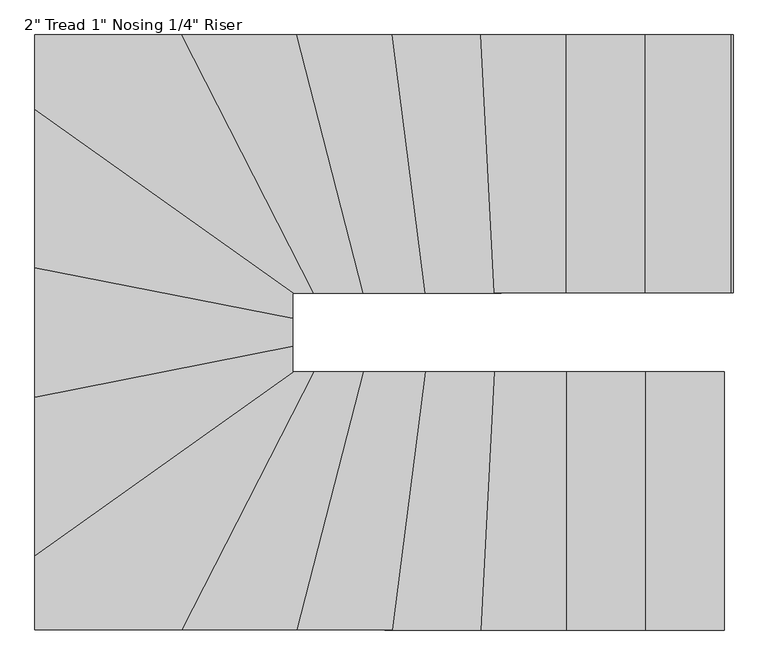
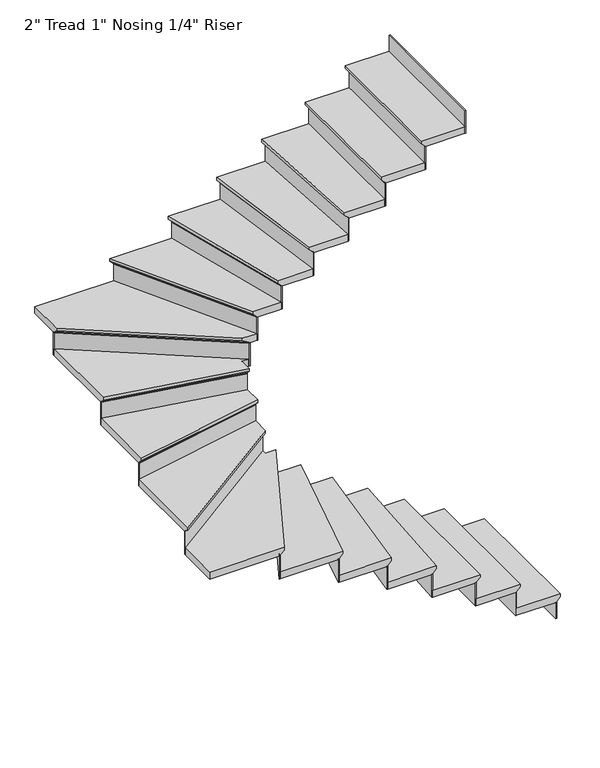
"""IFC4 building model written with IfcOpenShell, lengths in millimetres: stair flight geometry."""

from ifc_helpers import new_model, si_unit, origin, place, context, project, spatial, faceted_brep, source, transform, mapped, element, save


def stair_flight_b82eb699(model_context):
    return source(origin(), model_context, "Body", "Brep", [
        faceted_brep([(-8198.7117747, 8373.1716937, 150.2833333), (-8198.7117747, 8373.1716937, 169.3333333), (-8198.7117747, 7458.7716937, 169.3333333), (-8198.7117747, 7458.7716937, 150.2833333), (-8224.1117747, 8373.1716937, 124.8833333), (-8224.1117747, 7458.7716937, 124.8833333), (-8503.5117747, 8373.1716937, 169.3333333), (-8503.5117747, 7458.7716937, 169.3333333), (-8224.1117747, 7458.7716937, 118.5333333), (-8503.5117747, 7458.7716937, 118.5333333), (-8503.5117747, 8373.1716937, 118.5333333), (-8224.1117747, 8373.1716937, 118.5333333)], [[[0, 1, 2, 3]], [[4, 0, 3, 5]], [[2, 1, 6, 7]], [[8, 9, 10, 11]], [[2, 7, 9, 8, 5, 3]], [[8, 11, 4, 5]], [[6, 1, 0, 4, 11, 10]], [[7, 6, 10, 9]]]),
        faceted_brep([(-8224.1117747, 8373.1716937, 118.5333333), (-8224.1117747, 8373.1716937, 0.0), (-8230.4617747, 8373.1716937, 0.0), (-8230.4617747, 8373.1716937, 118.5333333), (-8224.1117747, 7458.7716937, 118.5333333), (-8230.4617747, 7458.7716937, 118.5333333), (-8230.4617747, 7458.7716937, 0.0), (-8224.1117747, 7458.7716937, 0.0)], [[[0, 1, 2, 3]], [[4, 5, 6, 7]], [[1, 0, 4, 7]], [[2, 1, 7, 6]], [[3, 2, 6, 5]], [[0, 3, 5, 4]]]),
        faceted_brep([(-8503.5117747, 8373.1716937, 287.8666667), (-8503.5117747, 8373.1716937, 118.5333333), (-8509.8617747, 8373.1716937, 118.5333333), (-8509.8617747, 8373.1716937, 287.8666667), (-8503.5117747, 7458.7716937, 287.8666667), (-8509.8617747, 7458.7716937, 287.8666667), (-8509.8617747, 7458.7716937, 118.5333333), (-8503.5117747, 7458.7716937, 118.5333333)], [[[0, 1, 2, 3]], [[4, 5, 6, 7]], [[1, 0, 4, 7]], [[2, 1, 7, 6]], [[3, 2, 6, 5]], [[0, 3, 5, 4]]]),
        faceted_brep([(-8478.1117747, 7458.7716937, 338.6666667), (-8478.1117747, 8373.1716937, 338.6666667), (-8782.9117747, 8373.1716937, 338.6666667), (-8782.9117747, 7458.7716937, 338.6666667), (-8503.5117747, 7458.7716937, 287.8666667), (-8782.9117747, 7458.7716937, 287.8666667), (-8782.9117747, 8373.1716937, 287.8666667), (-8503.5117747, 8373.1716937, 287.8666667), (-8503.5117747, 7458.7716937, 294.2166667), (-8478.1117747, 7458.7716937, 319.6166667), (-8503.5117747, 8373.1716937, 294.2166667), (-8478.1117747, 8373.1716937, 319.6166667)], [[[0, 1, 2, 3]], [[4, 5, 6, 7]], [[0, 3, 5, 4, 8, 9]], [[4, 7, 10, 8]], [[2, 1, 11, 10, 7, 6]], [[3, 2, 6, 5]], [[11, 1, 0, 9]], [[10, 11, 9, 8]]]),
        faceted_brep([(-8782.9117747, 8373.1716937, 457.2), (-8782.9117747, 8373.1716937, 287.8666667), (-8789.2617747, 8373.1716937, 287.8666667), (-8789.2617747, 8373.1716937, 457.2), (-8782.9117747, 7458.7716937, 457.2), (-8789.2617747, 7458.7716937, 457.2), (-8789.2617747, 7458.7716937, 287.8666667), (-8782.9117747, 7458.7716937, 287.8666667)], [[[0, 1, 2, 3]], [[4, 5, 6, 7]], [[1, 0, 4, 7]], [[2, 1, 7, 6]], [[3, 2, 6, 5]], [[0, 3, 5, 4]]]),
        faceted_brep([(-8757.5117747, 7458.7716937, 508.0), (-8757.5117747, 8373.1716937, 508.0), (-9038.5789362, 8373.1716937, 508.0), (-9086.1132066, 7458.7716937, 508.0), (-8782.9117747, 7458.7716937, 457.2), (-9086.1132066, 7458.7716937, 457.2), (-9038.5789362, 8373.1716937, 457.2), (-8782.9117747, 8373.1716937, 457.2), (-8782.9117747, 7458.7716937, 463.55), (-8757.5117747, 7458.7716937, 488.95), (-8782.9117747, 8373.1716937, 463.55), (-8757.5117747, 8373.1716937, 488.95)], [[[0, 1, 2, 3]], [[4, 5, 6, 7]], [[0, 3, 5, 4, 8, 9]], [[4, 7, 10, 8]], [[2, 1, 11, 10, 7, 6]], [[3, 2, 6, 5]], [[11, 1, 0, 9]], [[10, 11, 9, 8]]]),
        faceted_brep([(-9038.5789362, 8373.1716937, 626.5333333), (-9038.5789362, 8373.1716937, 457.2), (-9044.9375104, 8373.1716937, 457.2), (-9044.9375104, 8373.1716937, 626.5333333), (-9086.1132066, 7458.7716937, 626.5333333), (-9092.4717808, 7458.7716937, 626.5333333), (-9092.4717808, 7458.7716937, 457.2), (-9086.1132066, 7458.7716937, 457.2)], [[[0, 1, 2, 3]], [[4, 5, 6, 7]], [[1, 0, 4, 7]], [[2, 1, 7, 6]], [[3, 2, 6, 5]], [[0, 3, 5, 4]]]),
        faceted_brep([(-9060.67891, 7458.7716937, 677.3333333), (-9013.1446395, 8373.1716937, 677.3333333), (-9282.745636, 8373.1716937, 677.3333333), (-9401.1016877, 7458.7716937, 677.3333333), (-9086.1132066, 7458.7716937, 626.5333333), (-9401.1016877, 7458.7716937, 626.5333333), (-9282.745636, 8373.1716937, 626.5333333), (-9038.5789362, 8373.1716937, 626.5333333), (-9086.1132066, 7458.7716937, 632.8833333), (-9060.67891, 7458.7716937, 658.2833333), (-9038.5789362, 8373.1716937, 632.8833333), (-9013.1446395, 8373.1716937, 658.2833333)], [[[0, 1, 2, 3]], [[4, 5, 6, 7]], [[0, 3, 5, 4, 8, 9]], [[4, 7, 10, 8]], [[2, 1, 11, 10, 7, 6]], [[3, 2, 6, 5]], [[11, 1, 0, 9]], [[10, 11, 9, 8]]]),
        faceted_brep([(-9282.745636, 8373.1716937, 795.8666667), (-9282.745636, 8373.1716937, 626.5333333), (-9289.1486078, 8373.1716937, 626.5333333), (-9289.1486078, 8373.1716937, 795.8666667), (-9401.1016877, 7458.7716937, 795.8666667), (-9407.5046595, 7458.7716937, 795.8666667), (-9407.5046595, 7458.7716937, 626.5333333), (-9401.1016877, 7458.7716937, 626.5333333)], [[[0, 1, 2, 3]], [[4, 5, 6, 7]], [[1, 0, 4, 7]], [[2, 1, 7, 6]], [[3, 2, 6, 5]], [[0, 3, 5, 4]]]),
        faceted_brep([(-9375.4898006, 7458.7716937, 846.6666667), (-9257.1337489, 8373.1716937, 846.6666667), (-9504.3728585, 8373.1716937, 846.6666667), (-9739.5033059, 7458.7716937, 846.6666667), (-9401.1016877, 7458.7716937, 795.8666667), (-9739.5033059, 7458.7716937, 795.8666667), (-9504.3728585, 8373.1716937, 795.8666667), (-9282.745636, 8373.1716937, 795.8666667), (-9401.1016877, 7458.7716937, 802.2166667), (-9375.4898006, 7458.7716937, 827.6166667), (-9282.745636, 8373.1716937, 802.2166667), (-9257.1337489, 8373.1716937, 827.6166667)], [[[0, 1, 2, 3]], [[4, 5, 6, 7]], [[0, 3, 5, 4, 8, 9]], [[4, 7, 10, 8]], [[2, 1, 11, 10, 7, 6]], [[3, 2, 6, 5]], [[11, 1, 0, 9]], [[10, 11, 9, 8]]]),
        faceted_brep([(-9504.3728585, 8373.1716937, 965.2), (-9504.3728585, 8373.1716937, 795.8666667), (-9510.9294354, 8373.1716937, 795.8666667), (-9510.9294354, 8373.1716937, 965.2), (-9739.5033059, 7458.7716937, 965.2), (-9746.0598828, 7458.7716937, 965.2), (-9746.0598828, 7458.7716937, 795.8666667), (-9739.5033059, 7458.7716937, 795.8666667)], [[[0, 1, 2, 3]], [[4, 5, 6, 7]], [[1, 0, 4, 7]], [[2, 1, 7, 6]], [[3, 2, 6, 5]], [[0, 3, 5, 4]]]),
        faceted_brep([(-9713.2769985, 7458.7716937, 1016.0), (-9478.146551, 8373.1716937, 1016.0), (-9680.7194946, 8373.1716937, 1016.0), (-10149.5441159, 7458.7716937, 1016.0), (-9739.5033059, 7458.7716937, 965.2), (-10149.5441159, 7458.7716937, 965.2), (-9680.7194946, 8373.1716937, 965.2), (-9504.3728585, 8373.1716937, 965.2), (-9739.5033059, 7458.7716937, 971.55), (-9713.2769985, 7458.7716937, 996.95), (-9504.3728585, 8373.1716937, 971.55), (-9478.146551, 8373.1716937, 996.95)], [[[0, 1, 2, 3]], [[4, 5, 6, 7]], [[0, 3, 5, 4, 8, 9]], [[4, 7, 10, 8]], [[2, 1, 11, 10, 7, 6]], [[3, 2, 6, 5]], [[11, 1, 0, 9]], [[10, 11, 9, 8]]]),
        faceted_brep([(-9680.7194946, 8373.1716937, 1134.5333333), (-9680.7194946, 8373.1716937, 965.2), (-9687.8554777, 8373.1716937, 965.2), (-9687.8554777, 8373.1716937, 1134.5333333), (-10149.5441159, 7458.7716937, 1134.5333333), (-10156.6800991, 7458.7716937, 1134.5333333), (-10156.6800991, 7458.7716937, 965.2), (-10149.5441159, 7458.7716937, 965.2)], [[[0, 1, 2, 3]], [[4, 5, 6, 7]], [[1, 0, 4, 7]], [[2, 1, 7, 6]], [[3, 2, 6, 5]], [[0, 3, 5, 4]]]),
        faceted_brep([(-10640.8434666, 7752.4528274, 1185.3333333), (-10640.8434666, 7458.7716937, 1185.3333333), (-10121.0001834, 7458.7716937, 1185.3333333), (-9652.1755621, 8373.1716937, 1185.3333333), (-9726.4434666, 8373.1716937, 1185.3333333), (-9726.4434666, 8402.7267766, 1185.3333333), (-10640.8434666, 7458.7716937, 1134.5333333), (-10640.8434666, 7752.4528274, 1134.5333333), (-9726.4434666, 8402.7267766, 1134.5333333), (-9726.4434666, 8373.1716937, 1134.5333333), (-9680.7194946, 8373.1716937, 1134.5333333), (-10149.5441159, 7458.7716937, 1134.5333333), (-10149.5441159, 7458.7716937, 1140.8833333), (-10121.0001834, 7458.7716937, 1166.2833333), (-9680.7194946, 8373.1716937, 1140.8833333), (-9652.1755621, 8373.1716937, 1166.2833333)], [[[0, 1, 2, 3, 4, 5]], [[6, 7, 8, 9, 10, 11]], [[1, 0, 7, 6]], [[2, 1, 6, 11, 12, 13]], [[11, 10, 14, 12]], [[4, 3, 15, 14, 10, 9]], [[5, 4, 9, 8]], [[0, 5, 8, 7]], [[15, 3, 2, 13]], [[14, 15, 13, 12]]]),
        faceted_brep([(-9726.4434666, 8402.7267766, 1303.8666667), (-9726.4434666, 8402.7267766, 1134.5333333), (-9726.4434666, 8410.5187513, 1134.5333333), (-9726.4434666, 8410.5187513, 1303.8666667), (-10640.8434666, 7752.4528274, 1303.8666667), (-10640.8434666, 7760.2448022, 1303.8666667), (-10640.8434666, 7760.2448022, 1134.5333333), (-10640.8434666, 7752.4528274, 1134.5333333)], [[[0, 1, 2, 3]], [[4, 5, 6, 7]], [[1, 0, 4, 7]], [[2, 1, 7, 6]], [[3, 2, 6, 5]], [[0, 3, 5, 4]]]),
        faceted_brep([(-10640.8434666, 7721.2849282, 1354.6666667), (-9726.4434666, 8371.5588774, 1354.6666667), (-9726.4434666, 8489.1808636, 1354.6666667), (-10640.8434666, 8308.9400073, 1354.6666667), (-10640.8434666, 7752.4528274, 1303.8666667), (-10640.8434666, 8308.9400073, 1303.8666667), (-9726.4434666, 8489.1808636, 1303.8666667), (-9726.4434666, 8402.7267766, 1303.8666667), (-10640.8434666, 7752.4528274, 1310.2166667), (-10640.8434666, 7721.2849282, 1335.6166667), (-9726.4434666, 8402.7267766, 1310.2166667), (-9726.4434666, 8371.5588774, 1335.6166667)], [[[0, 1, 2, 3]], [[4, 5, 6, 7]], [[0, 3, 5, 4, 8, 9]], [[4, 7, 10, 8]], [[2, 1, 11, 10, 7, 6]], [[3, 2, 6, 5]], [[11, 1, 0, 9]], [[10, 11, 9, 8]]]),
        faceted_brep([(-9726.4434666, 8489.1808636, 1473.2), (-9726.4434666, 8489.1808636, 1303.8666667), (-9726.4434666, 8495.6530491, 1303.8666667), (-9726.4434666, 8495.6530491, 1473.2), (-10640.8434666, 8308.9400073, 1473.2), (-10640.8434666, 8315.4121927, 1473.2), (-10640.8434666, 8315.4121927, 1303.8666667), (-10640.8434666, 8308.9400073, 1303.8666667)], [[[0, 1, 2, 3]], [[4, 5, 6, 7]], [[1, 0, 4, 7]], [[2, 1, 7, 6]], [[3, 2, 6, 5]], [[0, 3, 5, 4]]]),
        faceted_brep([(-10640.8434666, 8283.0512655, 1524.0), (-9726.4434666, 8463.2921219, 1524.0), (-9726.4434666, 8588.3400073, 1524.0), (-10640.8434666, 8768.5808636, 1524.0), (-10640.8434666, 8308.9400073, 1473.2), (-10640.8434666, 8768.5808636, 1473.2), (-9726.4434666, 8588.3400073, 1473.2), (-9726.4434666, 8489.1808636, 1473.2), (-10640.8434666, 8308.9400073, 1479.55), (-10640.8434666, 8283.0512655, 1504.95), (-9726.4434666, 8489.1808636, 1479.55), (-9726.4434666, 8463.2921219, 1504.95)], [[[0, 1, 2, 3]], [[4, 5, 6, 7]], [[0, 3, 5, 4, 8, 9]], [[4, 7, 10, 8]], [[2, 1, 11, 10, 7, 6]], [[3, 2, 6, 5]], [[11, 1, 0, 9]], [[10, 11, 9, 8]]]),
        faceted_brep([(-9726.4434666, 8588.3400073, 1642.5333333), (-9726.4434666, 8588.3400073, 1473.2), (-9726.4434666, 8594.8121927, 1473.2), (-9726.4434666, 8594.8121927, 1642.5333333), (-10640.8434666, 8768.5808636, 1642.5333333), (-10640.8434666, 8775.0530491, 1642.5333333), (-10640.8434666, 8775.0530491, 1473.2), (-10640.8434666, 8768.5808636, 1473.2)], [[[0, 1, 2, 3]], [[4, 5, 6, 7]], [[1, 0, 4, 7]], [[2, 1, 7, 6]], [[3, 2, 6, 5]], [[0, 3, 5, 4]]]),
        faceted_brep([(-10640.8434666, 8742.6921219, 1693.3333333), (-9726.4434666, 8562.4512655, 1693.3333333), (-9726.4434666, 8652.5716937, 1693.3333333), (-9680.3479921, 8652.5716937, 1693.3333333), (-10640.8434666, 9335.6263584, 1693.3333333), (-10640.8434666, 8768.5808636, 1642.5333333), (-10640.8434666, 9335.6263584, 1642.5333333), (-9680.3479921, 8652.5716937, 1642.5333333), (-9726.4434666, 8652.5716937, 1642.5333333), (-9726.4434666, 8588.3400073, 1642.5333333), (-10640.8434666, 8768.5808636, 1648.8833333), (-10640.8434666, 8742.6921219, 1674.2833333), (-9726.4434666, 8588.3400073, 1648.8833333), (-9726.4434666, 8562.4512655, 1674.2833333)], [[[0, 1, 2, 3, 4]], [[5, 6, 7, 8, 9]], [[0, 4, 6, 5, 10, 11]], [[5, 9, 12, 10]], [[2, 1, 13, 12, 9, 8]], [[3, 2, 8, 7]], [[4, 3, 7, 6]], [[13, 1, 0, 11]], [[12, 13, 11, 10]]]),
        faceted_brep([(-9680.3479921, 8652.5716937, 1811.8666667), (-9680.3479921, 8652.5716937, 1642.5333333), (-9669.3910996, 8652.5716937, 1642.5333333), (-9669.3910996, 8652.5716937, 1811.8666667), (-10640.8434666, 9335.6263584, 1811.8666667), (-10640.8434666, 9343.4183332, 1811.8666667), (-10640.8434666, 9343.4183332, 1642.5333333), (-10640.8434666, 9335.6263584, 1642.5333333)], [[[0, 1, 2, 3]], [[4, 5, 6, 7]], [[1, 0, 4, 7]], [[2, 1, 7, 6]], [[3, 2, 6, 5]], [[0, 3, 5, 4]]]),
        faceted_brep([(-10092.4562509, 9566.9716937, 1862.6666667), (-10640.8434666, 9566.9716937, 1862.6666667), (-10640.8434666, 9304.4584592, 1862.6666667), (-9724.1755621, 8652.5716937, 1862.6666667), (-9623.6316295, 8652.5716937, 1862.6666667), (-10640.8434666, 9566.9716937, 1811.8666667), (-10092.4562509, 9566.9716937, 1811.8666667), (-9623.6316295, 8652.5716937, 1811.8666667), (-9680.3479921, 8652.5716937, 1811.8666667), (-10640.8434666, 9335.6263584, 1811.8666667), (-10640.8434666, 9335.6263584, 1818.2166667), (-10640.8434666, 9304.4584592, 1843.6166667), (-9680.3479921, 8652.5716937, 1818.2166667), (-9724.1755621, 8652.5716937, 1843.6166667)], [[[0, 1, 2, 3, 4]], [[5, 6, 7, 8, 9]], [[1, 0, 6, 5]], [[2, 1, 5, 9, 10, 11]], [[9, 8, 12, 10]], [[4, 3, 13, 12, 8, 7]], [[0, 4, 7, 6]], [[13, 3, 2, 11]], [[12, 13, 11, 10]]]),
        faceted_brep([(-9623.6316295, 8652.5716937, 1981.2), (-9623.6316295, 8652.5716937, 1811.8666667), (-9616.4956464, 8652.5716937, 1811.8666667), (-9616.4956464, 8652.5716937, 1981.2), (-10092.4562509, 9566.9716937, 1981.2), (-10085.3202677, 9566.9716937, 1981.2), (-10085.3202677, 9566.9716937, 1811.8666667), (-10092.4562509, 9566.9716937, 1811.8666667)], [[[0, 1, 2, 3]], [[4, 5, 6, 7]], [[1, 0, 4, 7]], [[2, 1, 7, 6]], [[3, 2, 6, 5]], [[0, 3, 5, 4]]]),
        faceted_brep([(-10121.0001834, 9566.9716937, 2032.0), (-9652.1755621, 8652.5716937, 2032.0), (-9451.9202436, 8652.5716937, 2032.0), (-9687.050691, 9566.9716937, 2032.0), (-10092.4562509, 9566.9716937, 1981.2), (-9687.050691, 9566.9716937, 1981.2), (-9451.9202436, 8652.5716937, 1981.2), (-9623.6316295, 8652.5716937, 1981.2), (-10092.4562509, 9566.9716937, 1987.55), (-10121.0001834, 9566.9716937, 2012.95), (-9623.6316295, 8652.5716937, 1987.55), (-9652.1755621, 8652.5716937, 2012.95)], [[[0, 1, 2, 3]], [[4, 5, 6, 7]], [[0, 3, 5, 4, 8, 9]], [[4, 7, 10, 8]], [[2, 1, 11, 10, 7, 6]], [[3, 2, 6, 5]], [[11, 1, 0, 9]], [[10, 11, 9, 8]]]),
        faceted_brep([(-9451.9202436, 8652.5716937, 2150.5333333), (-9451.9202436, 8652.5716937, 1981.2), (-9445.3636667, 8652.5716937, 1981.2), (-9445.3636667, 8652.5716937, 2150.5333333), (-9687.050691, 9566.9716937, 2150.5333333), (-9680.4941141, 9566.9716937, 2150.5333333), (-9680.4941141, 9566.9716937, 1981.2), (-9687.050691, 9566.9716937, 1981.2)], [[[0, 1, 2, 3]], [[4, 5, 6, 7]], [[1, 0, 4, 7]], [[2, 1, 7, 6]], [[3, 2, 6, 5]], [[0, 3, 5, 4]]]),
        faceted_brep([(-9713.2769985, 9566.9716937, 2201.3333333), (-9478.146551, 8652.5716937, 2201.3333333), (-9231.5218618, 8652.5716937, 2201.3333333), (-9349.8779135, 9566.9716937, 2201.3333333), (-9687.050691, 9566.9716937, 2150.5333333), (-9349.8779135, 9566.9716937, 2150.5333333), (-9231.5218618, 8652.5716937, 2150.5333333), (-9451.9202436, 8652.5716937, 2150.5333333), (-9687.050691, 9566.9716937, 2156.8833333), (-9713.2769985, 9566.9716937, 2182.2833333), (-9451.9202436, 8652.5716937, 2156.8833333), (-9478.146551, 8652.5716937, 2182.2833333)], [[[0, 1, 2, 3]], [[4, 5, 6, 7]], [[0, 3, 5, 4, 8, 9]], [[4, 7, 10, 8]], [[2, 1, 11, 10, 7, 6]], [[3, 2, 6, 5]], [[11, 1, 0, 9]], [[10, 11, 9, 8]]]),
        faceted_brep([(-9231.5218618, 8652.5716937, 2319.8666667), (-9231.5218618, 8652.5716937, 2150.5333333), (-9225.11889, 8652.5716937, 2150.5333333), (-9225.11889, 8652.5716937, 2319.8666667), (-9349.8779135, 9566.9716937, 2319.8666667), (-9343.4749417, 9566.9716937, 2319.8666667), (-9343.4749417, 9566.9716937, 2150.5333333), (-9349.8779135, 9566.9716937, 2150.5333333)], [[[0, 1, 2, 3]], [[4, 5, 6, 7]], [[1, 0, 4, 7]], [[2, 1, 7, 6]], [[3, 2, 6, 5]], [[0, 3, 5, 4]]]),
        faceted_brep([(-9375.4898006, 9566.9716937, 2370.6666667), (-9257.1337489, 8652.5716937, 2370.6666667), (-8987.7103429, 8652.5716937, 2370.6666667), (-9035.2446133, 9566.9716937, 2370.6666667), (-9349.8779135, 9566.9716937, 2319.8666667), (-9035.2446133, 9566.9716937, 2319.8666667), (-8987.7103429, 8652.5716937, 2319.8666667), (-9231.5218618, 8652.5716937, 2319.8666667), (-9349.8779135, 9566.9716937, 2326.2166667), (-9375.4898006, 9566.9716937, 2351.6166667), (-9231.5218618, 8652.5716937, 2326.2166667), (-9257.1337489, 8652.5716937, 2351.6166667)], [[[0, 1, 2, 3]], [[4, 5, 6, 7]], [[0, 3, 5, 4, 8, 9]], [[4, 7, 10, 8]], [[2, 1, 11, 10, 7, 6]], [[3, 2, 6, 5]], [[11, 1, 0, 9]], [[10, 11, 9, 8]]]),
        faceted_brep([(-8987.7103429, 8652.5716937, 2489.2), (-8987.7103429, 8652.5716937, 2319.8666667), (-8981.3517687, 8652.5716937, 2319.8666667), (-8981.3517687, 8652.5716937, 2489.2), (-9035.2446133, 9566.9716937, 2489.2), (-9028.8860391, 9566.9716937, 2489.2), (-9028.8860391, 9566.9716937, 2319.8666667), (-9035.2446133, 9566.9716937, 2319.8666667)], [[[0, 1, 2, 3]], [[4, 5, 6, 7]], [[1, 0, 4, 7]], [[2, 1, 7, 6]], [[3, 2, 6, 5]], [[0, 3, 5, 4]]]),
        faceted_brep([(-9060.67891, 9566.9716937, 2540.0), (-9013.1446395, 8652.5716937, 2540.0), (-8732.1117747, 8652.5716937, 2540.0), (-8732.1117747, 9566.9716937, 2540.0), (-9035.2446133, 9566.9716937, 2489.2), (-8732.1117747, 9566.9716937, 2489.2), (-8732.1117747, 8652.5716937, 2489.2), (-8987.7103429, 8652.5716937, 2489.2), (-9035.2446133, 9566.9716937, 2495.55), (-9060.67891, 9566.9716937, 2520.95), (-8987.7103429, 8652.5716937, 2495.55), (-9013.1446395, 8652.5716937, 2520.95)], [[[0, 1, 2, 3]], [[4, 5, 6, 7]], [[0, 3, 5, 4, 8, 9]], [[4, 7, 10, 8]], [[2, 1, 11, 10, 7, 6]], [[3, 2, 6, 5]], [[11, 1, 0, 9]], [[10, 11, 9, 8]]]),
        faceted_brep([(-8732.1117747, 8652.5716937, 2658.5333333), (-8732.1117747, 8652.5716937, 2489.2), (-8725.7617747, 8652.5716937, 2489.2), (-8725.7617747, 8652.5716937, 2658.5333333), (-8732.1117747, 9566.9716937, 2658.5333333), (-8725.7617747, 9566.9716937, 2658.5333333), (-8725.7617747, 9566.9716937, 2489.2), (-8732.1117747, 9566.9716937, 2489.2)], [[[0, 1, 2, 3]], [[4, 5, 6, 7]], [[1, 0, 4, 7]], [[2, 1, 7, 6]], [[3, 2, 6, 5]], [[0, 3, 5, 4]]]),
        faceted_brep([(-8757.5117747, 9566.9716937, 2709.3333333), (-8757.5117747, 8652.5716937, 2709.3333333), (-8452.7117747, 8652.5716937, 2709.3333333), (-8452.7117747, 9566.9716937, 2709.3333333), (-8732.1117747, 9566.9716937, 2658.5333333), (-8452.7117747, 9566.9716937, 2658.5333333), (-8452.7117747, 8652.5716937, 2658.5333333), (-8732.1117747, 8652.5716937, 2658.5333333), (-8732.1117747, 9566.9716937, 2664.8833333), (-8757.5117747, 9566.9716937, 2690.2833333), (-8732.1117747, 8652.5716937, 2664.8833333), (-8757.5117747, 8652.5716937, 2690.2833333)], [[[0, 1, 2, 3]], [[4, 5, 6, 7]], [[0, 3, 5, 4, 8, 9]], [[4, 7, 10, 8]], [[2, 1, 11, 10, 7, 6]], [[3, 2, 6, 5]], [[11, 1, 0, 9]], [[10, 11, 9, 8]]]),
        faceted_brep([(-8452.7117747, 8652.5716937, 2827.8666667), (-8452.7117747, 8652.5716937, 2658.5333333), (-8446.3617747, 8652.5716937, 2658.5333333), (-8446.3617747, 8652.5716937, 2827.8666667), (-8452.7117747, 9566.9716937, 2827.8666667), (-8446.3617747, 9566.9716937, 2827.8666667), (-8446.3617747, 9566.9716937, 2658.5333333), (-8452.7117747, 9566.9716937, 2658.5333333)], [[[0, 1, 2, 3]], [[4, 5, 6, 7]], [[1, 0, 4, 7]], [[2, 1, 7, 6]], [[3, 2, 6, 5]], [[0, 3, 5, 4]]]),
        faceted_brep([(-8173.3117747, 8652.5716937, 2997.2), (-8173.3117747, 8652.5716937, 2827.8666667), (-8166.9617747, 8652.5716937, 2827.8666667), (-8166.9617747, 8652.5716937, 2997.2), (-8173.3117747, 9566.9716937, 2997.2), (-8166.9617747, 9566.9716937, 2997.2), (-8166.9617747, 9566.9716937, 2827.8666667), (-8173.3117747, 9566.9716937, 2827.8666667)], [[[0, 1, 2, 3]], [[4, 5, 6, 7]], [[1, 0, 4, 7]], [[2, 1, 7, 6]], [[3, 2, 6, 5]], [[0, 3, 5, 4]]]),
        faceted_brep([(-8478.1117747, 9566.9716937, 2878.6666667), (-8478.1117747, 8652.5716937, 2878.6666667), (-8173.3117747, 8652.5716937, 2878.6666667), (-8173.3117747, 9566.9716937, 2878.6666667), (-8452.7117747, 9566.9716937, 2827.8666667), (-8173.3117747, 9566.9716937, 2827.8666667), (-8173.3117747, 8652.5716937, 2827.8666667), (-8452.7117747, 8652.5716937, 2827.8666667), (-8452.7117747, 9566.9716937, 2834.2166667), (-8478.1117747, 9566.9716937, 2859.6166667), (-8452.7117747, 8652.5716937, 2834.2166667), (-8478.1117747, 8652.5716937, 2859.6166667)], [[[0, 1, 2, 3]], [[4, 5, 6, 7]], [[0, 3, 5, 4, 8, 9]], [[4, 7, 10, 8]], [[2, 1, 11, 10, 7, 6]], [[3, 2, 6, 5]], [[11, 1, 0, 9]], [[10, 11, 9, 8]]]),
    ])


if __name__ == "__main__":
    model = new_model("IFC4")
    model_context = context("Model", 3, world=origin())
    ifc_project = project(units=[si_unit("LENGTHUNIT", "METRE", prefix="MILLI")], contexts=[model_context])
    site = spatial("IfcSite", under=ifc_project)
    building = spatial("IfcBuilding", under=site)
    placement = place(None, origin())
    stair_flight_shape = stair_flight_b82eb699(model_context)
    element("IfcStairFlight", 1, ObjectType="2\" Tread 1\" Nosing 1/4\" Riser", at=placement, inside=building, context=model_context, shape_type="MappedRepresentation", body=[
        mapped(stair_flight_shape, transform((0.0, 0.0, 0.0), x_axis=(1.0, 0.0, 0.0), y_axis=(0.0, 1.0, 0.0), z_axis=(0.0, 0.0, 1.0))),
    ])
    save(model, "model.ifc")
